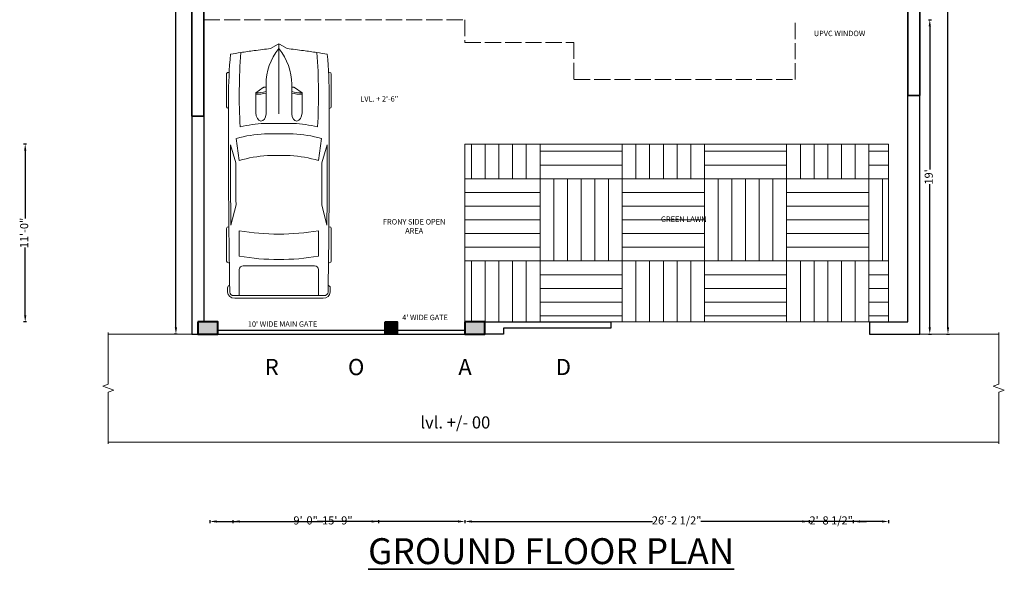
# Model space of a CAD drawing. Units: inches. Extents: x 2845 to 3575, y 808 to 1996.
# Tile 1 of 6: x 2845 to 3575, y 808 to 1215. Entities that reach past the tile are written whole.
import ezdxf

# ---------------------------------------------------------------- set-up
doc = ezdxf.new("R2010")
doc.units = ezdxf.units.IN
doc.linetypes.add('ACAD_ISO02W100', pattern=[15, 12, -3])
for name, color, linetype, lineweight in [('A-ANNO-DIMS', 2, 'Continuous', 18), ('A-ANNO-SYMB', 7, 'Continuous', 18), ('A-ANNO-TEXT', 7, 'Continuous', 18), ('A-ANNO-TITL', 7, 'Continuous', 35), ('A-AREA-IDEN', 7, 'Continuous', 18), ('A-COLS', 7, 'Continuous', 40), ('A-ROOF-OVHD', 7, 'ACAD_ISO02W100', 18), ('A-WALL', 1, 'Continuous', 35), ('C-PRKG-VEHI', 8, 'Continuous', 13), ('C-PROP', 7, 'Continuous', 30), ('C-ROAD', 7, 'Continuous', 18), ('C-SITE-GATE', 4, 'Continuous', 25), ('L-PLNT-BEDS', 3, 'Continuous', 18), ('L-PLNT-PATT', 3, 'Continuous', 13)]:
    doc.layers.add(name, color=color, linetype=linetype, lineweight=lineweight)
doc.styles.get("Standard").update_dxf_attribs({"font": 'arial.ttf'})
doc.dimstyles.new('ISO-25', dxfattribs={"dimtxt": 6, "dimasz": 5, "dimexe": 1.25, "dimexo": 0.625, "dimtad": 0, "dimlunit": 4, "dimtxsty": 'Standard', "dimcen": 2.5, "dimclrd": 1, "dimclre": 1, "dimclrt": 1, "dimadec": 0, "dimazin": 0, "dimtfac": 1, "dimtmove": 0, "dimatfit": 3, "dimfxl": 1, "dimfxlon": 1, "dimfrac": 1, "dimarcsym": 0})

# ---------------------------------------------------------------- blocks, each defined once
blk = doc.blocks.new('*U21')
for p, q in [((21.1, 37.41), (21.1, 36.83)), ((46.55, 38.89), (22.35, 38.89)), ((47.8, 37.39), (47.8, 37.41)), ((135.45, 37.07), (135.45, 37.41)), ((136.7, 38.89), (160.9, 38.89)), ((162.15, 37.41), (162.15, 36.77)), ((70.03, 31.54), (86.41, 29.35)), ((87.99, 31.87), (74.76, 35.92)), ((134.31, 35.6), (119.29, 31.78)), ((138.42, 29.35), (157.25, 29.35)), ((186.47, 29.35), (167.01, 29.35)), ((186.47, -33.5), (186.47, 33.5)), ((188.4, -32.76), (188.4, 32.76)), ((164.52, 26.39), (164.52, -26.39)), ((32.27, 11.63), (36.13, 17.17)), ((36.13, 17.17), (50.94, 17.17)), ((29.77, 9.51), (51.68, 9.51)), ((32.12, 9.51), (32.12, 11.15)), ((58.92, -10.77), (58.92, 10.77)), ((66.55, -10.53), (66.55, 10.53)), ((82.74, 8.5), (82.74, -8.5)), ((186.47, -10.53), (186.47, 10.53)), ((3.27, 6.13), (0.1, 0.41)), ((0, 0), (51.68, 0)), ((0.1, -0.41), (3.27, -6.13)), ((29.77, -9.51), (51.68, -9.51)), ((32.12, -9.51), (32.12, -11.15)), ((32.27, -11.63), (36.13, -17.17)), ((36.13, -17.17), (50.94, -17.17)), ((86.41, -29.35), (70.03, -31.54)), ((87.99, -31.87), (74.76, -35.92)), ((134.31, -35.6), (119.29, -31.78)), ((157.25, -29.35), (138.42, -29.35)), ((167.01, -29.35), (186.47, -29.35)), ((21.1, -37.41), (21.1, -36.83)), ((46.55, -38.89), (22.35, -38.89)), ((47.8, -37.39), (47.8, -37.41)), ((135.45, -37.07), (135.45, -37.41)), ((136.7, -38.89), (160.9, -38.89)), ((162.15, -37.41), (162.15, -36.77))]:
    blk.add_line(p, q)
for centre, major_axis, ratio, start_param, end_param in [((41.19, -490.86), (0, 528.23), 0.842304, 0.00281, 0.075598), ((22.35, 37.41), (0, -1.48), 0.842304, 3.141593, 4.712389), ((64.48, -10555.62), (0, 10593.03), 0.842304, -0.013397, 0.002797), ((46.55, 37.41), (0, 1.48), 0.842304, -1.570796, 0), ((136.7, 37.41), (0, -1.48), 0.842304, 3.141593, 4.712389), ((160.9, 37.41), (0, 1.48), 0.842304, -1.570796, 0), ((180.63, 35.84), (0, 2.22), 0.842304, -0.013017, 1.249894), ((64.48, -10556.36), (0, 10595.31), 0.842304, -0.013397, -0.013017), ((183.98, 32.76), (0, -5.25), 0.842304, 1.570796, 3.128196), ((266.03, -27.52), (0, 313.31), 0.842304, 1.367076, 1.39176), ((37.47, -593.96), (0, -623.33), 0.842304, 3.096046, 3.200911), ((135.29, 5.39), (0, 81.77), 0.842304, 1.245306, 1.50788), ((64.48, -10555.62), (0, -10591.55), 0.842304, 3.133765, 3.140441), ((149.6, 2.8), (0, -79.58), 0.842304, 4.372215, 4.640744), ((95.79, -3666.35), (0, -3698.24), 0.842304, 3.134049, 3.144098), ((17.08, 0), (0, 147.02), 0.842304, 4.511394, 4.913384), ((35.91, 0), (0, 147.02), 0.842304, 4.511394, 4.913384), ((167.01, 26.39), (0, 2.96), 0.842304, 0, 1.570796), ((183.98, 33.5), (0, -2.96), 0.842304, 1.570796, 3.128196), ((259.18, -27.52), (0, -305.3), 0.842304, 4.528606, 4.561838), ((134.4, 5.39), (0, -89.78), 0.842304, 4.449482, 4.652344), ((-204.49, 52.4), (0, -250.96), 0.842304, 1.385369, 1.434372), ((13.04, 17.01), (0, 27.42), 0.842304, 4.435146, 4.718221), ((14.2, 17.01), (0, 27.42), 0.842304, 4.435146, 4.718221), ((50.79, 13.34), (6.34, -0.36), 0.603834, -1.395552, 1.581315), ((29.77, -46.66), (0, 56.17), 0.842304, 0, 0.590319), ((32.75, 11.15), (0, 0.74), 0.842304, 0.879714, 1.570796), ((0.62, 0), (0, -0.74), 0.842304, 4.131459, 5.293319), ((-204.49, -52.4), (0, 250.96), 0.842304, -1.434372, -1.385369), ((29.77, 46.66), (0, 56.17), 0.842304, 2.551274, 3.141593), ((32.75, -11.15), (0, -0.74), 0.842304, 4.712389, 5.403472), ((13.04, -17.01), (0, -27.42), 0.842304, 1.564964, 1.848039), ((14.2, -17.01), (0, -27.42), 0.842304, 1.564964, 1.848039), ((134.4, -5.39), (0, -89.78), 0.842304, -1.510751, -1.307889), ((135.29, -5.39), (0, -81.77), 0.842304, -1.50788, -1.245306), ((149.6, -2.8), (0, -79.58), 0.842304, -1.499151, -1.230623), ((259.18, 27.52), (0, 305.3), 0.842304, 1.721348, 1.754579), ((266.03, 27.52), (0, 313.31), 0.842304, 1.749832, 1.774517), ((37.47, 593.96), (0, -623.33), 0.842304, -0.059319, 0.045547), ((167.01, -26.39), (0, -2.96), 0.842304, 4.712389, 6.283185), ((41.19, 490.86), (0, -528.23), 0.842304, -0.075598, -0.00281), ((64.48, 10555.62), (0, 10593.03), 0.842304, 3.138796, 3.15499), ((64.48, 10555.62), (0, -10591.55), 0.842304, 0.001152, 0.007828), ((95.79, 3666.35), (0, -3698.24), 0.842304, -0.002505, 0.007544), ((183.98, -33.5), (0, 2.96), 0.842304, 3.15499, 4.712389), ((183.98, -32.76), (0, -5.25), 0.842304, 0.013397, 1.570796), ((22.35, -37.41), (0, 1.48), 0.842304, 1.570796, 3.141593), ((46.55, -37.41), (0, -1.48), 0.842304, 0, 1.570796), ((136.7, -37.41), (0, -1.48), 0.842304, -1.570796, 0), ((160.9, -37.41), (0, 1.48), 0.842304, 3.141593, 4.712389), ((180.63, -35.84), (0, -2.22), 0.842304, -1.249894, 0.013017), ((64.48, 10556.36), (0, 10595.31), 0.842304, 3.15461, 3.15499)]:
    blk.add_ellipse(centre, major_axis=major_axis, ratio=ratio, start_param=start_param, end_param=end_param)
at = {"extrusion": (0, 0, -1)}
blk.add_ellipse((50.79, -13.34), major_axis=(6.34, 0.36), ratio=0.603834, start_param=-1.395552, end_param=1.581315, dxfattribs=at)
blk = doc.blocks.new('*D28')
at = {"layer": 'A-ANNO-DIMS', "color": 0, "lineweight": -2, "transparency": 16777216}
for p, q in [((3518.95, 1215.17), (3521.2, 1215.17)), ((3519.95, 1210.17), (3519.95, 1104.11)), ((3519.95, 987.17), (3519.95, 1093.24)), ((3518.95, 982.17), (3521.2, 982.17))]:
    blk.add_line(p, q, dxfattribs=at)
at = {"layer": 'A-ANNO-DIMS', "color": 0, "transparency": 16777216}
for points in [[(3519.11, 1210.17), (3520.78, 1210.17), (3519.95, 1215.17)], [(3519.11, 987.17), (3520.78, 987.17), (3519.95, 982.17)]]:
    blk.add_solid(points, dxfattribs=at)
at = {"layer": 'Defpoints', "color": 0, "transparency": 16777216}
for p in [(3507.65, 1215.17), (3512.62, 982.17), (3519.95, 982.17)]:
    blk.add_point(p, dxfattribs=at)
at = {"layer": 'A-ANNO-DIMS', "color": 0, "transparency": 16777216, "insert": (3519.95, 1098.67), "char_height": 6, "attachment_point": 5, "rotation": 90}
blk.add_mtext("19'", dxfattribs=at)
blk = doc.blocks.new('*D29')
at = {"layer": 'A-ANNO-DIMS', "color": 0, "lineweight": -2, "transparency": 16777216}
for p, q in [((3532.44, 1925.07), (3534.69, 1925.07)), ((3533.44, 1920.07), (3533.44, 1464.53)), ((3533.44, 987.17), (3533.44, 1442.72)), ((3532.44, 982.17), (3534.69, 982.17))]:
    blk.add_line(p, q, dxfattribs=at)
at = {"layer": 'A-ANNO-DIMS', "color": 0, "transparency": 16777216}
for points in [[(3532.6, 1920.07), (3534.27, 1920.07), (3533.44, 1925.07)], [(3532.6, 987.17), (3534.27, 987.17), (3533.44, 982.17)]]:
    blk.add_solid(points, dxfattribs=at)
at = {"layer": 'Defpoints', "color": 0, "transparency": 16777216}
for p in [(3519.95, 1925.07), (3533.44, 1925.07), (3512.62, 982.17)]:
    blk.add_point(p, dxfattribs=at)
at = {"layer": 'A-ANNO-DIMS', "color": 0, "transparency": 16777216, "insert": (3533.44, 1453.62), "char_height": 6, "attachment_point": 5, "rotation": 90}
blk.add_mtext('78\'-7"', dxfattribs=at)
blk = doc.blocks.new('*D30')
at = {"layer": 'A-ANNO-DIMS', "color": 0, "lineweight": -2, "transparency": 16777216}
for p, q in [((2961.94, 1929.67), (2959.69, 1929.67)), ((2960.94, 1924.67), (2960.94, 1473.45)), ((2960.94, 987.17), (2960.94, 1438.39)), ((2961.94, 982.17), (2959.69, 982.17))]:
    blk.add_line(p, q, dxfattribs=at)
at = {"layer": 'A-ANNO-DIMS', "color": 0, "transparency": 16777216}
for points in [[(2960.11, 1924.67), (2961.77, 1924.67), (2960.94, 1929.67)], [(2960.11, 987.17), (2961.77, 987.17), (2960.94, 982.17)]]:
    blk.add_solid(points, dxfattribs=at)
at = {"layer": 'Defpoints', "color": 0, "transparency": 16777216}
for p in [(2972.62, 1929.67), (2960.94, 982.17), (2972.62, 982.17)]:
    blk.add_point(p, dxfattribs=at)
at = {"layer": 'A-ANNO-DIMS', "color": 0, "transparency": 16777216, "insert": (2960.94, 1455.92), "char_height": 6, "attachment_point": 5, "rotation": 90}
blk.add_mtext('78\'-11{\\H1x;\\S1#2;}"', dxfattribs=at)
blk = doc.blocks.new('COL-15x9')
h = blk.add_hatch(color=256)
h.dxf.hatch_style = 1
h.paths.add_polyline_path([(15, 9), (0, 9), (0, 0), (15, 0)])
blk.add_lwpolyline([(0, 9), (0, 0), (15, 0), (15, 9)], close=True)
blk = doc.blocks.new('COL-9x9')
h = blk.add_hatch(color=256)
h.dxf.hatch_style = 1
h.paths.add_polyline_path([(9, 9), (0, 9), (0, 0), (9, 0)])
blk.add_lwpolyline([(0, 9), (9, 9), (9, 0), (0, 0)], close=True)
blk = doc.blocks.new('BREAK-ROAD')
blk.add_lwpolyline([(4.12, 82.59), (4.12, 44.29), (0, 42.79), (8.24, 39.79), (4.12, 38.29), (4.12, 0)])
blk = doc.blocks.new('*D71')
at = {"layer": 'A-ANNO-DIMS', "color": 1, "lineweight": -2, "transparency": 16777216}
for p, q in [((3175.12, 844.33), (3175.12, 842.08)), ((3180.12, 843.33), (3314.3, 843.33)), ((3484.43, 843.33), (3350.25, 843.33)), ((3489.43, 844.33), (3489.43, 842.08))]:
    blk.add_line(p, q, dxfattribs=at)
at = {"layer": 'A-ANNO-DIMS', "color": 1, "transparency": 16777216}
for points in [[(3180.12, 844.17), (3180.12, 842.5), (3175.12, 843.33)], [(3484.43, 844.17), (3484.43, 842.5), (3489.43, 843.33)]]:
    blk.add_solid(points, dxfattribs=at)
at = {"layer": 'Defpoints', "color": 0, "transparency": 16777216}
for p in [(3175.12, 991.17), (3489.43, 991.17), (3489.43, 843.33)]:
    blk.add_point(p, dxfattribs=at)
at = {"layer": 'A-ANNO-DIMS', "color": 1, "transparency": 16777216, "insert": (3332.27, 843.33), "char_height": 6, "attachment_point": 5}
blk.add_mtext('26\'-2 1/2"', dxfattribs=at)
blk = doc.blocks.new('*D72')
at = {"layer": 'A-ANNO-DIMS', "color": 1, "lineweight": -2, "transparency": 16777216}
for p, q in [((2850.17, 1123.03), (2847.92, 1123.03)), ((2849.17, 1118.03), (2849.17, 1067.75)), ((2849.17, 996.17), (2849.17, 1046.45)), ((2850.17, 991.17), (2847.92, 991.17))]:
    blk.add_line(p, q, dxfattribs=at)
at = {"layer": 'A-ANNO-DIMS', "color": 1, "transparency": 16777216}
for points in [[(2848.34, 1118.03), (2850.01, 1118.03), (2849.17, 1123.03)], [(2848.34, 996.17), (2850.01, 996.17), (2849.17, 991.17)]]:
    blk.add_solid(points, dxfattribs=at)
at = {"layer": 'Defpoints', "color": 0, "transparency": 16777216}
for p in [(2849.17, 1123.03), (3175.12, 1123.03), (3175.12, 991.17)]:
    blk.add_point(p, dxfattribs=at)
at = {"layer": 'A-ANNO-DIMS', "color": 1, "transparency": 16777216, "insert": (2849.17, 1057.1), "char_height": 6, "attachment_point": 5, "rotation": 90}
blk.add_mtext('11\'-0"', dxfattribs=at)
blk = doc.blocks.new('*D73')
at = {"layer": 'A-ANNO-DIMS', "color": 1, "lineweight": -2, "transparency": 16777216}
for p, q in [((2986.12, 844.33), (2986.12, 842.08)), ((2991.12, 843.33), (3069.97, 843.33)), ((3170.12, 843.33), (3091.26, 843.33)), ((3175.12, 844.33), (3175.12, 842.08))]:
    blk.add_line(p, q, dxfattribs=at)
at = {"layer": 'A-ANNO-DIMS', "color": 1, "transparency": 16777216}
for points in [[(2991.12, 844.17), (2991.12, 842.5), (2986.12, 843.33)], [(3170.12, 844.17), (3170.12, 842.5), (3175.12, 843.33)]]:
    blk.add_solid(points, dxfattribs=at)
at = {"layer": 'Defpoints', "color": 0, "transparency": 16777216}
for p in [(2986.12, 1250.42), (3175.12, 1252.17), (3175.12, 843.33)]:
    blk.add_point(p, dxfattribs=at)
at = {"layer": 'A-ANNO-DIMS', "color": 1, "transparency": 16777216, "insert": (3080.62, 843.33), "char_height": 6, "attachment_point": 5}
blk.add_mtext('15\'-9"', dxfattribs=at)
blk = doc.blocks.new('*D76')
at = {"layer": 'A-ANNO-DIMS', "color": 1, "lineweight": -2, "transparency": 16777216}
for p, q in [((3003.12, 844.33), (3003.12, 842.08)), ((3008.12, 843.33), (3048.52, 843.33)), ((3106.12, 843.33), (3065.72, 843.33)), ((3111.12, 844.33), (3111.12, 842.08))]:
    blk.add_line(p, q, dxfattribs=at)
at = {"layer": 'A-ANNO-DIMS', "color": 1, "transparency": 16777216}
for points in [[(3008.12, 844.17), (3008.12, 842.5), (3003.12, 843.33)], [(3106.12, 844.17), (3106.12, 842.5), (3111.12, 843.33)]]:
    blk.add_solid(points, dxfattribs=at)
at = {"layer": 'Defpoints', "color": 0, "transparency": 16777216}
for p in [(3003.12, 1441.17), (3111.12, 1441.17), (3111.12, 843.33)]:
    blk.add_point(p, dxfattribs=at)
at = {"layer": 'A-ANNO-DIMS', "color": 1, "transparency": 16777216, "insert": (3057.12, 843.33), "char_height": 6, "attachment_point": 5}
blk.add_mtext('9\'-0"', dxfattribs=at)
blk = doc.blocks.new('*D77')
at = {"layer": 'A-ANNO-DIMS', "color": 1, "lineweight": -2, "transparency": 16777216}
for p, q in [((3425.54, 843.33), (3420.54, 843.33)), ((3430.54, 844.33), (3430.54, 842.08)), ((3430.54, 843.33), (3431.19, 843.33)), ((3463.12, 843.33), (3462.47, 843.33)), ((3463.12, 844.33), (3463.12, 842.08)), ((3468.12, 843.33), (3473.12, 843.33))]:
    blk.add_line(p, q, dxfattribs=at)
at = {"layer": 'A-ANNO-DIMS', "color": 1, "transparency": 16777216}
for points in [[(3425.54, 844.17), (3425.54, 842.5), (3430.54, 843.33)], [(3468.12, 844.17), (3468.12, 842.5), (3463.12, 843.33)]]:
    blk.add_solid(points, dxfattribs=at)
at = {"layer": 'Defpoints', "color": 0, "transparency": 16777216}
for p in [(3430.54, 1215.17), (3463.12, 1215.17), (3463.12, 843.33)]:
    blk.add_point(p, dxfattribs=at)
at = {"layer": 'A-ANNO-DIMS', "color": 1, "transparency": 16777216, "insert": (3446.83, 843.33), "char_height": 6, "attachment_point": 5}
blk.add_mtext('2\'-8 1/2"', dxfattribs=at)

msp = doc.modelspace()

# ---------------------------------------------------------------- hatches: boundary and pattern name
at = {"layer": 'L-PLNT-PATT'}
h = msp.add_hatch(dxfattribs=at)
h.set_pattern_fill('AR-PARQ1', color=256, scale=0.2)
h.paths.add_polyline_path([(3175.116, 1123.027), (3175.116, 991.173), (3190.116, 991.173), (3283.505, 991.173), (3489.433, 991.173), (3489.433, 1123.027)])
h.paths.add_polyline_path([(3319.304, 1063.128), (3358.873, 1063.128), (3358.873, 1071.371), (3319.304, 1071.371)], flags=24)

# ---------------------------------------------------------------- linework, layer by layer
at = {"layer": 'A-ROOF-OVHD'}
for p, q in [((2981.616, 1214.969), (3175.116, 1214.969)), ((3175.116, 1214.969), (3175.116, 1198.244)), ((3420.121, 1170.861), (3420.121, 1215.173)), ((3175.116, 1198.244), (3256.116, 1198.244)), ((3256.116, 1198.244), (3256.116, 1170.861)), ((3256.116, 1170.861), (3420.121, 1170.861))]:
    msp.add_line(p, q, dxfattribs=at)
at = {"layer": 'A-WALL'}
for p, q in [((2972.616, 1798.173), (2972.616, 1143.734)), ((3512.616, 1159.066), (3512.616, 1798.173)), ((2981.616, 1441.173), (2981.616, 1143.734)), ((3503.616, 1159.066), (3503.616, 1356.173)), ((3503.616, 1159.066), (3512.616, 1159.066)), ((2972.616, 1143.734), (2981.616, 1143.734))]:
    msp.add_line(p, q, dxfattribs=at)
at = {"layer": 'C-PROP'}
for p, q in [((3503.616, 991.173), (3503.616, 1159.066)), ((3512.616, 982.173), (3512.616, 1159.066)), ((2981.616, 1143.734), (2981.616, 991.173)), ((2981.616, 991.173), (2992.116, 991.173)), ((3115.985, 991.173), (3124.985, 991.173)), ((3175.116, 991.173), (3190.116, 991.173)), ((3190.116, 991.173), (3283.505, 991.173)), ((3283.505, 986.573), (3203.751, 986.573)), ((3203.751, 986.573), (3203.751, 982.173)), ((3283.505, 991.173), (3283.505, 986.573)), ((3475.251, 991.173), (3475.251, 982.173)), ((3475.251, 991.173), (3503.616, 991.173)), ((3203.751, 982.173), (3190.116, 982.173))]:
    msp.add_line(p, q, dxfattribs=at)
for points in [[(2972.616, 1143.734), (2972.616, 982.173), (2992.116, 982.173)], [(3115.985, 982.173), (3124.985, 982.173)], [(3175.116, 982.173), (3190.116, 982.173)], [(3475.251, 982.173), (3512.616, 982.173)]]:
    msp.add_lwpolyline(points, dxfattribs=at)
at = {"layer": 'C-ROAD'}
for p, q in [((2972.616, 982.173), (2910.793, 982.173)), ((3512.616, 982.173), (3571.1, 982.173)), ((2910.793, 902.085), (3571.1, 902.085))]:
    msp.add_line(p, q, dxfattribs=at)
at = {"layer": 'C-SITE-GATE'}
for p, q in [((2992.116, 985.173), (3115.985, 985.173)), ((2992.116, 982.173), (3115.985, 982.173)), ((3124.985, 985.173), (3175.116, 985.173)), ((3124.985, 982.173), (3175.116, 982.173))]:
    msp.add_line(p, q, dxfattribs=at)
at = {"layer": 'L-PLNT-BEDS'}
for p, q in [((3175.116, 991.173), (3175.116, 1123.027)), ((3175.116, 1123.027), (3489.433, 1123.027)), ((3489.433, 1123.027), (3489.433, 991.173)), ((3489.433, 991.173), (3283.505, 991.173))]:
    msp.add_line(p, q, dxfattribs=at)

# ---------------------------------------------------------------- block references
at = {"layer": 'A-ANNO-SYMB', "rotation": 180}
for p in [(2914.914, 983.423), (3575.221, 983.423)]:
    msp.add_blockref('BREAK-ROAD', p, dxfattribs=at)
at = {"layer": 'A-COLS'}
for name, p in [('COL-15x9', (2977.116, 982.173)), ('COL-9x9', (3115.985, 982.173)), ('COL-15x9', (3175.116, 982.173))]:
    msp.add_blockref(name, p, dxfattribs=at)
at = {"layer": 'C-PRKG-VEHI', "rotation": 270}
msp.add_blockref('*U21', (3037.272, 1197.185), dxfattribs=at)

# ---------------------------------------------------------------- texts
at = {"layer": 'A-ANNO-SYMB', "attachment_point": 1}
for s, width, insert, char_height in [('LVL. + 2\'-6"', 45.255, (3097.661, 1158.469), 4), ('lvl. +/- 00', 143.54042, (3142.227, 921.228), 9)]:
    msp.add_mtext_dynamic_manual_height_columns(s, width=width, gutter_width=12.5, heights=[0], dxfattribs=dict(at, insert=insert, char_height=char_height))
at = {"layer": 'A-ANNO-TEXT', "char_height": 4, "attachment_point": 1}
for s, width, insert in [('UPVC WINDOW', 45.255, (3433.964, 1206.998)), ("4' WIDE GATE", 40.64723, (3128.77, 996.526)), ("10' WIDE MAIN GATE", 72.28832, (3014.275, 991.642))]:
    msp.add_mtext_dynamic_manual_height_columns(s, width=width, gutter_width=12.5, heights=[0], dxfattribs=dict(at, insert=insert))
at = {"layer": 'A-ANNO-TITL', "insert": (3103.424, 830.932), "char_height": 19.2, "attachment_point": 1}
msp.add_mtext_dynamic_manual_height_columns('{\\fArial|b1|i0|c0|p34;\\LGROUND FLOOR PLAN}', width=351.3943, gutter_width=12.5, heights=[0], dxfattribs=at)
at = {"layer": 'A-AREA-IDEN', "attachment_point": 1}
for s, width, insert, char_height in [('\\pxqc;FRONY SIDE OPEN AREA', 54.59778, (3110.311, 1067.402), 4), ('GREEN LAWN', 46.5647, (3320.601, 1069.38), 4), ('R              O                   A                 D', 298.41711, (3026.776, 963.79), 12)]:
    msp.add_mtext_dynamic_manual_height_columns(s, width=width, gutter_width=12.5, heights=[0], dxfattribs=dict(at, insert=insert, char_height=char_height))

# ---------------------------------------------------------------- dimensions: what is measured, and where the dimension line sits
at = {"layer": 'A-ANNO-DIMS'}
for base, p1, p2, override, picture, middle in [((2960.94, 982.173), (2972.616, 1929.673), (2972.616, 982.173), {"dimclrd": 0, "dimclre": 0, "dimclrt": 0}, '*D30', (2960.94, 1455.923)), ((3533.438, 1925.073), (3512.616, 982.173), (3519.947, 1925.073), {"dimclrd": 0, "dimclre": 0, "dimclrt": 0}, '*D29', (3533.438, 1453.623)), ((2849.172, 1123.027), (3175.116, 991.173), (3175.116, 1123.027), {"dimdec": 1, "dimlfac": 1, "dimrnd": 0, "dimzin": 1, "dimdsep": 46, "dimlunit": 4, "dimfrac": 2}, '*D72', (2849.172, 1057.1))]:
    dim = msp.add_linear_dim(base=base, p1=p1, p2=p2, angle=90, dimstyle='ISO-25', override=override, dxfattribs=at)
    dim.commit()
    dim.dimension.update_dxf_attribs({"geometry": picture, "text_midpoint": middle})
for base, p1, p2, picture, middle in [((3111.116, 843.335), (3003.116, 1441.173), (3111.116, 1441.173), '*D76', (3057.116, 843.335)), ((3175.116, 843.335), (2986.116, 1250.417), (3175.116, 1252.173), '*D73', (3080.616, 843.335)), ((3463.116, 843.335), (3430.545, 1215.173), (3463.116, 1215.173), '*D77', (3446.83, 843.335)), ((3489.433, 843.335), (3175.116, 991.173), (3489.433, 991.173), '*D71', (3332.274, 843.335))]:
    dim = msp.add_linear_dim(base=base, p1=p1, p2=p2, dimstyle='ISO-25', override={"dimdec": 1, "dimlfac": 1, "dimrnd": 0, "dimzin": 1, "dimdsep": 46, "dimlunit": 4, "dimfrac": 2}, dxfattribs=at)
    dim.commit()
    dim.dimension.update_dxf_attribs({"geometry": picture, "text_midpoint": middle})
dim = msp.add_linear_dim(base=(3519.947, 982.173), p1=(3507.652, 1215.173), p2=(3512.616, 982.173), angle=90, text="19'", dimstyle='ISO-25', override={"dimclrd": 0, "dimclre": 0, "dimclrt": 0, "dimtmove": 1}, dxfattribs=at)
dim.commit()
dim.dimension.update_dxf_attribs({"geometry": '*D28', "text_midpoint": (3519.947, 1098.673)})

doc.saveas('drawing.dxf')
